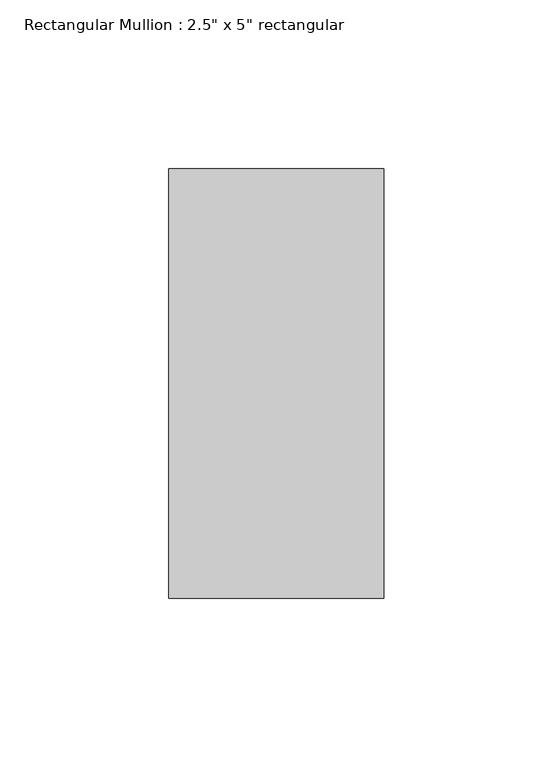
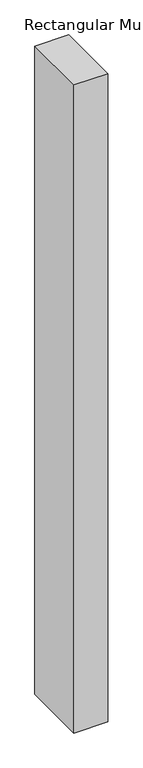
"""IFC4 building model written with IfcOpenShell, lengths in millimetres: member geometry."""

from ifc_helpers import new_model, si_unit, frame, origin, place, context, project, spatial, polyline, outline, extrude, source, transform, mapped, element, save


def member_b9a8557f(model_context):
    return source(origin(), model_context, "Body", "SweptSolid", [
        extrude(outline(polyline([(31.75, 63.5), (31.75, -63.5), (-31.75, -63.5), (-31.75, 63.5), (31.75, 63.5)])), frame((0.0, 0.0, -1288.9615505), z_axis=(0.0, 0.0, 1.0), x_axis=(1.0, 0.0, 0.0)), (0.0, 0.0, 1.0), 1288.9615505),
    ])


if __name__ == "__main__":
    model = new_model("IFC4")
    model_context = context("Model", 3, world=origin())
    ifc_project = project(units=[si_unit("LENGTHUNIT", "METRE", prefix="MILLI")], contexts=[model_context])
    site = spatial("IfcSite", under=ifc_project)
    building = spatial("IfcBuilding", under=site)
    placement = place(None, origin())
    member_shape = member_b9a8557f(model_context)
    element("IfcMember", 1, ObjectType="Rectangular Mullion : 2.5\" x 5\" rectangular", at=placement, inside=building, context=model_context, shape_type="MappedRepresentation", body=[
        mapped(member_shape, transform((0.0, 0.0, 0.0), x_axis=(1.0, 0.0, 0.0), y_axis=(0.0, 1.0, 0.0), z_axis=(0.0, 0.0, 1.0))),
    ])
    save(model, "model.ifc")

# Revit data of these elements
# Type "Rectangular Mullion : 2.5\" x 5\" rectangular"
#   built-in parameter 1007304 = 0.416667 (stored number, unit not read)
#   built-in parameter 1007301 = 0.104167 (stored number, unit not read)
#   built-in parameter 1007300 = 0.104167 (stored number, unit not read)
# Element 1 (IfcMember, "Rectangular Mullion : 2.5\" x 5\" rectangular")
#   Materials on its faces: "Aluminum"
# Materials
#   "Aluminum": class "Metal", colour RGB 247 247 247, transparency 0, Description = "Aluminum 6061", Cost = 0
